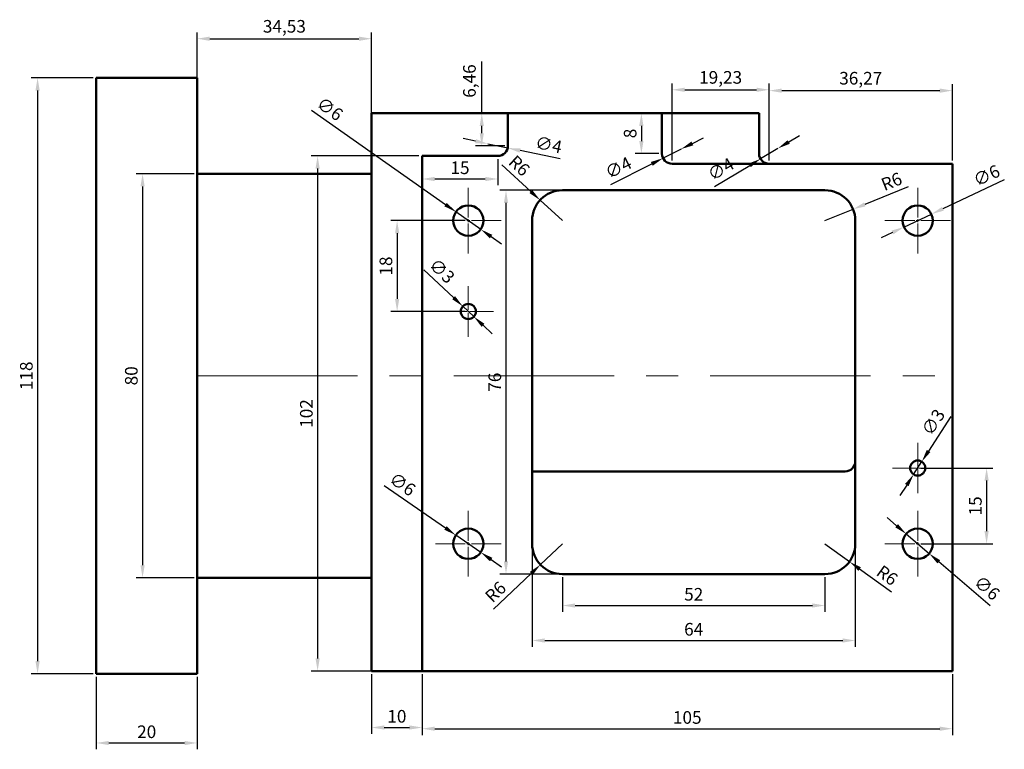
# Model space of a CAD drawing. Units: millimetres. Extents: x 1194 to 1920, y 1729 to 2086.
# Tile 3 of 5: x 1494 to 1689, y 1729 to 1874. Entities that reach past the tile are written whole.
import ezdxf

# ---------------------------------------------------------------- set-up
doc = ezdxf.new("R2010")
doc.units = ezdxf.units.MM
doc.linetypes.add('CENTER', pattern=[50.8, 31.75, -6.35, 6.35, -6.35])
for name, color, linetype, lineweight in [('M-CNTR', 1, 'CENTER', 18), ('M-DIMS', 2, 'Continuous', 25), ('M-OUTL', 7, 'Continuous', 50)]:
    doc.layers.add(name, color=color, linetype=linetype, lineweight=lineweight)
doc.styles.get("Standard").update_dxf_attribs({"font": 'arial.ttf'})
doc.dimstyles.new('ISO-25', dxfattribs={"dimtxt": 2.5, "dimasz": 2.5, "dimexe": 1.25, "dimexo": 0.625, "dimtad": 1, "dimtxsty": 'Standard', "dimcen": 2.5, "dimadec": 0, "dimazin": 0, "dimtfac": 1, "dimtmove": 0, "dimatfit": 3, "dimfxl": 1, "dimarcsym": 0})

# ---------------------------------------------------------------- blocks, each defined once
blk = doc.blocks.new('*D101')
at = {"layer": 'Defpoints', "color": 0, "transparency": 16777216}
for p in [(1509.24, 1862.41), (1497.63, 1744.41), (1509.24, 1744.41)]:
    blk.add_point(p, dxfattribs=at)
at = {"layer": 'M-DIMS', "color": 0, "lineweight": -2, "transparency": 16777216}
for p, q in [((1508.62, 1862.41), (1496.38, 1862.41)), ((1497.63, 1859.91), (1497.63, 1746.91)), ((1508.62, 1744.41), (1496.38, 1744.41))]:
    blk.add_line(p, q, dxfattribs=at)
at = {"layer": 'M-DIMS', "color": 0, "transparency": 16777216}
for points in [[(1497.22, 1859.91), (1498.05, 1859.91), (1497.63, 1862.41)], [(1497.22, 1746.91), (1498.05, 1746.91), (1497.63, 1744.41)]]:
    blk.add_solid(points, dxfattribs=at)
at = {"layer": 'M-DIMS', "color": 0, "transparency": 16777216, "insert": (1495.73, 1803.41), "char_height": 2.5, "attachment_point": 5, "rotation": 90}
blk.add_mtext('118', dxfattribs=at)
blk = doc.blocks.new('*D102')
at = {"layer": 'Defpoints', "color": 0, "transparency": 16777216}
for p in [(1509.24, 1744.41), (1529.24, 1744.41), (1529.24, 1730.7)]:
    blk.add_point(p, dxfattribs=at)
at = {"layer": 'M-DIMS', "color": 0, "lineweight": -2, "transparency": 16777216}
for p, q in [((1509.24, 1743.78), (1509.24, 1729.45)), ((1529.24, 1743.78), (1529.24, 1729.45)), ((1511.74, 1730.7), (1526.74, 1730.7))]:
    blk.add_line(p, q, dxfattribs=at)
at = {"layer": 'M-DIMS', "color": 0, "transparency": 16777216}
for points in [[(1511.74, 1731.11), (1511.74, 1730.28), (1509.24, 1730.7)], [(1526.74, 1731.11), (1526.74, 1730.28), (1529.24, 1730.7)]]:
    blk.add_solid(points, dxfattribs=at)
at = {"layer": 'M-DIMS', "color": 0, "transparency": 16777216, "insert": (1519.24, 1732.6), "char_height": 2.5, "attachment_point": 5}
blk.add_mtext('20', dxfattribs=at)
blk = doc.blocks.new('*D103')
at = {"layer": 'Defpoints', "color": 0, "transparency": 16777216}
for p in [(1563.78, 1870.17), (1529.24, 1843.41), (1563.78, 1843.41)]:
    blk.add_point(p, dxfattribs=at)
at = {"layer": 'M-DIMS', "color": 0, "lineweight": -2, "transparency": 16777216}
for p, q in [((1529.24, 1844.03), (1529.24, 1871.42)), ((1531.74, 1870.17), (1561.28, 1870.17)), ((1563.78, 1844.03), (1563.78, 1871.42))]:
    blk.add_line(p, q, dxfattribs=at)
at = {"layer": 'M-DIMS', "color": 0, "transparency": 16777216}
for points in [[(1531.74, 1870.59), (1531.74, 1869.75), (1529.24, 1870.17)], [(1561.28, 1870.59), (1561.28, 1869.75), (1563.78, 1870.17)]]:
    blk.add_solid(points, dxfattribs=at)
at = {"layer": 'M-DIMS', "color": 0, "transparency": 16777216, "insert": (1546.51, 1872.3), "char_height": 2.5, "attachment_point": 5}
blk.add_mtext('34,53', dxfattribs=at)
blk = doc.blocks.new('*D104')
at = {"layer": 'Defpoints', "color": 0, "transparency": 16777216}
for p in [(1529.24, 1843.41), (1518.42, 1763.41), (1529.24, 1763.41)]:
    blk.add_point(p, dxfattribs=at)
at = {"layer": 'M-DIMS', "color": 0, "lineweight": -2, "transparency": 16777216}
for p, q in [((1528.62, 1843.41), (1517.17, 1843.41)), ((1518.42, 1840.91), (1518.42, 1765.91)), ((1528.62, 1763.41), (1517.17, 1763.41))]:
    blk.add_line(p, q, dxfattribs=at)
at = {"layer": 'M-DIMS', "color": 0, "transparency": 16777216}
for points in [[(1518.01, 1840.91), (1518.84, 1840.91), (1518.42, 1843.41)], [(1518.01, 1765.91), (1518.84, 1765.91), (1518.42, 1763.41)]]:
    blk.add_solid(points, dxfattribs=at)
at = {"layer": 'M-DIMS', "color": 0, "transparency": 16777216, "insert": (1516.52, 1803.41), "char_height": 2.5, "attachment_point": 5, "rotation": 90}
blk.add_mtext('80', dxfattribs=at)
blk = doc.blocks.new('*D105')
at = {"layer": 'Defpoints', "color": 0, "transparency": 16777216}
for p in [(1563.78, 1744.95), (1573.78, 1744.95), (1573.78, 1733.76)]:
    blk.add_point(p, dxfattribs=at)
at = {"layer": 'M-DIMS', "color": 0, "lineweight": -2, "transparency": 16777216}
for p, q in [((1563.78, 1744.32), (1563.78, 1732.51)), ((1573.78, 1744.32), (1573.78, 1732.51)), ((1566.28, 1733.76), (1571.28, 1733.76))]:
    blk.add_line(p, q, dxfattribs=at)
at = {"layer": 'M-DIMS', "color": 0, "transparency": 16777216}
for points in [[(1566.28, 1734.18), (1566.28, 1733.35), (1563.78, 1733.76)], [(1571.28, 1734.18), (1571.28, 1733.35), (1573.78, 1733.76)]]:
    blk.add_solid(points, dxfattribs=at)
at = {"layer": 'M-DIMS', "color": 0, "transparency": 16777216, "insert": (1568.78, 1735.66), "char_height": 2.5, "attachment_point": 5}
blk.add_mtext('10', dxfattribs=at)
blk = doc.blocks.new('*D106')
at = {"layer": 'Defpoints', "color": 0, "transparency": 16777216}
for p in [(1573.78, 1744.95), (1678.78, 1744.95), (1678.78, 1733.53)]:
    blk.add_point(p, dxfattribs=at)
at = {"layer": 'M-DIMS', "color": 0, "lineweight": -2, "transparency": 16777216}
for p, q in [((1573.78, 1744.32), (1573.78, 1732.28)), ((1678.78, 1744.32), (1678.78, 1732.28)), ((1576.28, 1733.53), (1676.28, 1733.53))]:
    blk.add_line(p, q, dxfattribs=at)
at = {"layer": 'M-DIMS', "color": 0, "transparency": 16777216}
for points in [[(1576.28, 1733.95), (1576.28, 1733.11), (1573.78, 1733.53)], [(1676.28, 1733.95), (1676.28, 1733.11), (1678.78, 1733.53)]]:
    blk.add_solid(points, dxfattribs=at)
at = {"layer": 'M-DIMS', "color": 0, "transparency": 16777216, "insert": (1626.28, 1735.43), "char_height": 2.5, "attachment_point": 5}
blk.add_mtext('105', dxfattribs=at)
blk = doc.blocks.new('*D107')
at = {"layer": 'Defpoints', "color": 0, "transparency": 16777216}
for p in [(1573.78, 1846.95), (1553.08, 1744.95), (1573.78, 1744.95)]:
    blk.add_point(p, dxfattribs=at)
at = {"layer": 'M-DIMS', "color": 0, "lineweight": -2, "transparency": 16777216}
for p, q in [((1573.15, 1846.95), (1551.83, 1846.95)), ((1553.08, 1844.45), (1553.08, 1747.45)), ((1573.15, 1744.95), (1551.83, 1744.95))]:
    blk.add_line(p, q, dxfattribs=at)
at = {"layer": 'M-DIMS', "color": 0, "transparency": 16777216}
for points in [[(1552.67, 1844.45), (1553.5, 1844.45), (1553.08, 1846.95)], [(1552.67, 1747.45), (1553.5, 1747.45), (1553.08, 1744.95)]]:
    blk.add_solid(points, dxfattribs=at)
at = {"layer": 'M-DIMS', "color": 0, "transparency": 16777216, "insert": (1551.18, 1795.95), "char_height": 2.5, "attachment_point": 5, "rotation": 90}
blk.add_mtext('102', dxfattribs=at)
blk = doc.blocks.new('*D108')
at = {"layer": 'Defpoints', "color": 0, "transparency": 16777216}
for p in [(1585.59, 1855.41), (1590.78, 1855.41), (1590.78, 1848.95)]:
    blk.add_point(p, dxfattribs=at)
at = {"layer": 'M-DIMS', "color": 0, "lineweight": -2, "transparency": 16777216}
for p, q in [((1585.59, 1855.41), (1585.59, 1865.66)), ((1590.15, 1855.41), (1584.34, 1855.41)), ((1585.59, 1851.45), (1585.59, 1852.91)), ((1590.15, 1848.95), (1584.34, 1848.95))]:
    blk.add_line(p, q, dxfattribs=at)
at = {"layer": 'M-DIMS', "color": 0, "transparency": 16777216}
for points in [[(1585.18, 1852.91), (1586.01, 1852.91), (1585.59, 1855.41)], [(1585.18, 1851.45), (1586.01, 1851.45), (1585.59, 1848.95)]]:
    blk.add_solid(points, dxfattribs=at)
at = {"layer": 'M-DIMS', "color": 0, "transparency": 16777216, "insert": (1583.47, 1861.79), "char_height": 2.5, "attachment_point": 5, "rotation": 90}
blk.add_mtext('6,46', dxfattribs=at)
blk = doc.blocks.new('*D109')
at = {"layer": 'Defpoints', "color": 0, "transparency": 16777216}
for p in [(1573.78, 1846.95), (1588.78, 1846.95), (1588.78, 1842.39)]:
    blk.add_point(p, dxfattribs=at)
at = {"layer": 'M-DIMS', "color": 0, "lineweight": -2, "transparency": 16777216}
for p, q in [((1573.78, 1846.32), (1573.78, 1841.14)), ((1588.78, 1846.32), (1588.78, 1841.14)), ((1576.28, 1842.39), (1586.28, 1842.39))]:
    blk.add_line(p, q, dxfattribs=at)
at = {"layer": 'M-DIMS', "color": 0, "transparency": 16777216}
for points in [[(1576.28, 1842.81), (1576.28, 1841.97), (1573.78, 1842.39)], [(1586.28, 1842.81), (1586.28, 1841.97), (1588.78, 1842.39)]]:
    blk.add_solid(points, dxfattribs=at)
at = {"layer": 'M-DIMS', "color": 0, "transparency": 16777216, "insert": (1581.28, 1844.29), "char_height": 2.5, "attachment_point": 5}
blk.add_mtext('15', dxfattribs=at)
blk = doc.blocks.new('*D110')
at = {"layer": 'Defpoints', "color": 0, "transparency": 16777216}
for p in [(1586.82, 1849.36), (1590.73, 1848.53)]:
    blk.add_point(p, dxfattribs=at)
at = {"layer": 'M-DIMS', "color": 0, "lineweight": -2, "transparency": 16777216}
for p, q in [((1584.37, 1849.87), (1581.93, 1850.39)), ((1586.82, 1849.36), (1590.73, 1848.53)), ((1601.11, 1846.35), (1593.18, 1848.02))]:
    blk.add_line(p, q, dxfattribs=at)
at = {"layer": 'M-DIMS', "color": 0, "transparency": 16777216}
for points in [[(1584.46, 1850.28), (1584.29, 1849.46), (1586.82, 1849.36)], [(1593.27, 1848.43), (1593.1, 1847.61), (1590.73, 1848.53)]]:
    blk.add_solid(points, dxfattribs=at)
at = {"layer": 'M-DIMS', "color": 0, "transparency": 16777216, "insert": (1598.77, 1848.86), "char_height": 2.5, "attachment_point": 5, "rotation": 348.1195}
blk.add_mtext('∅4', dxfattribs=at)
blk = doc.blocks.new('*D111')
at = {"layer": 'Defpoints', "color": 0, "transparency": 16777216}
for p in [(1621.49, 1846.51), (1625.06, 1848.31)]:
    blk.add_point(p, dxfattribs=at)
at = {"layer": 'M-DIMS', "color": 0, "lineweight": -2, "transparency": 16777216}
for p, q in [((1627.3, 1849.43), (1629.53, 1850.55)), ((1625.06, 1848.31), (1621.49, 1846.51)), ((1611.16, 1841.32), (1619.26, 1845.39))]:
    blk.add_line(p, q, dxfattribs=at)
at = {"layer": 'M-DIMS', "color": 0, "transparency": 16777216}
for points in [[(1627.11, 1849.8), (1627.49, 1849.06), (1625.06, 1848.31)], [(1619.07, 1845.76), (1619.44, 1845.01), (1621.49, 1846.51)]]:
    blk.add_solid(points, dxfattribs=at)
at = {"layer": 'M-DIMS', "color": 0, "transparency": 16777216, "insert": (1612.78, 1844.34), "char_height": 2.5, "attachment_point": 5, "rotation": 26.6783}
blk.add_mtext('∅4', dxfattribs=at)
blk = doc.blocks.new('*D112')
at = {"layer": 'Defpoints', "color": 0, "transparency": 16777216}
for p in [(1644.23, 1848.44), (1640.8, 1846.38)]:
    blk.add_point(p, dxfattribs=at)
at = {"layer": 'M-DIMS', "color": 0, "lineweight": -2, "transparency": 16777216}
for p, q in [((1646.37, 1849.72), (1648.52, 1851.01)), ((1644.23, 1848.44), (1640.8, 1846.38)), ((1631.71, 1840.93), (1638.65, 1845.09))]:
    blk.add_line(p, q, dxfattribs=at)
at = {"layer": 'M-DIMS', "color": 0, "transparency": 16777216}
for points in [[(1646.16, 1850.08), (1646.59, 1849.36), (1644.23, 1848.44)], [(1638.44, 1845.45), (1638.87, 1844.74), (1640.8, 1846.38)]]:
    blk.add_solid(points, dxfattribs=at)
at = {"layer": 'M-DIMS', "color": 0, "transparency": 16777216, "insert": (1633.09, 1844.06), "char_height": 2.5, "attachment_point": 5, "rotation": 30.9377}
blk.add_mtext('∅4', dxfattribs=at)
blk = doc.blocks.new('*D113')
at = {"layer": 'Defpoints', "color": 0, "transparency": 16777216}
for p in [(1621.28, 1855.41), (1617.2, 1847.41), (1621.28, 1847.41)]:
    blk.add_point(p, dxfattribs=at)
at = {"layer": 'M-DIMS', "color": 0, "lineweight": -2, "transparency": 16777216}
for p, q in [((1620.65, 1855.41), (1615.95, 1855.41)), ((1617.2, 1852.91), (1617.2, 1849.91)), ((1620.65, 1847.41), (1615.95, 1847.41))]:
    blk.add_line(p, q, dxfattribs=at)
at = {"layer": 'M-DIMS', "color": 0, "transparency": 16777216}
for points in [[(1616.78, 1852.91), (1617.62, 1852.91), (1617.2, 1855.41)], [(1616.78, 1849.91), (1617.62, 1849.91), (1617.2, 1847.41)]]:
    blk.add_solid(points, dxfattribs=at)
at = {"layer": 'M-DIMS', "color": 0, "transparency": 16777216, "insert": (1615.3, 1851.41), "char_height": 2.5, "attachment_point": 5, "rotation": 90}
blk.add_mtext('8', dxfattribs=at)
blk = doc.blocks.new('*D114')
at = {"layer": 'Defpoints', "color": 0, "transparency": 16777216}
for p in [(1642.51, 1860.06), (1623.28, 1845.41), (1642.51, 1845.41)]:
    blk.add_point(p, dxfattribs=at)
at = {"layer": 'M-DIMS', "color": 0, "lineweight": -2, "transparency": 16777216}
for p, q in [((1623.28, 1846.03), (1623.28, 1861.31)), ((1642.51, 1846.03), (1642.51, 1861.31)), ((1625.78, 1860.06), (1640.01, 1860.06))]:
    blk.add_line(p, q, dxfattribs=at)
at = {"layer": 'M-DIMS', "color": 0, "transparency": 16777216}
for points in [[(1625.78, 1860.48), (1625.78, 1859.64), (1623.28, 1860.06)], [(1640.01, 1860.48), (1640.01, 1859.64), (1642.51, 1860.06)]]:
    blk.add_solid(points, dxfattribs=at)
at = {"layer": 'M-DIMS', "color": 0, "transparency": 16777216, "insert": (1632.89, 1862.19), "char_height": 2.5, "attachment_point": 5}
blk.add_mtext('19,23', dxfattribs=at)
blk = doc.blocks.new('*D115')
at = {"layer": 'Defpoints', "color": 0, "transparency": 16777216}
for p in [(1678.78, 1859.89), (1642.51, 1845.41), (1678.78, 1845.41)]:
    blk.add_point(p, dxfattribs=at)
at = {"layer": 'M-DIMS', "color": 0, "lineweight": -2, "transparency": 16777216}
for p, q in [((1642.51, 1846.03), (1642.51, 1861.14)), ((1678.78, 1846.03), (1678.78, 1861.14)), ((1645.01, 1859.89), (1676.28, 1859.89))]:
    blk.add_line(p, q, dxfattribs=at)
at = {"layer": 'M-DIMS', "color": 0, "transparency": 16777216}
for points in [[(1645.01, 1860.31), (1645.01, 1859.47), (1642.51, 1859.89)], [(1676.28, 1860.31), (1676.28, 1859.47), (1678.78, 1859.89)]]:
    blk.add_solid(points, dxfattribs=at)
at = {"layer": 'M-DIMS', "color": 0, "transparency": 16777216, "insert": (1660.64, 1862.02), "char_height": 2.5, "attachment_point": 5}
blk.add_mtext('36,27', dxfattribs=at)
blk = doc.blocks.new('*D116')
at = {"layer": 'Defpoints', "color": 0, "transparency": 16777216}
for p in [(1601.56, 1764.15), (1653.56, 1764.15), (1653.56, 1757.92)]:
    blk.add_point(p, dxfattribs=at)
at = {"layer": 'M-DIMS', "color": 0, "lineweight": -2, "transparency": 16777216}
for p, q in [((1601.56, 1763.53), (1601.56, 1756.67)), ((1653.56, 1763.53), (1653.56, 1756.67)), ((1604.06, 1757.92), (1651.06, 1757.92))]:
    blk.add_line(p, q, dxfattribs=at)
at = {"layer": 'M-DIMS', "color": 0, "transparency": 16777216}
for points in [[(1604.06, 1758.34), (1604.06, 1757.51), (1601.56, 1757.92)], [(1651.06, 1758.34), (1651.06, 1757.51), (1653.56, 1757.92)]]:
    blk.add_solid(points, dxfattribs=at)
at = {"layer": 'M-DIMS', "color": 0, "transparency": 16777216, "insert": (1627.56, 1759.82), "char_height": 2.5, "attachment_point": 5}
blk.add_mtext('52', dxfattribs=at)
blk = doc.blocks.new('*D117')
at = {"layer": 'Defpoints', "color": 0, "transparency": 16777216}
for p in [(1595.56, 1770.15), (1659.56, 1770.15), (1659.56, 1751)]:
    blk.add_point(p, dxfattribs=at)
at = {"layer": 'M-DIMS', "color": 0, "lineweight": -2, "transparency": 16777216}
for p, q in [((1595.56, 1769.53), (1595.56, 1749.75)), ((1659.56, 1769.53), (1659.56, 1749.75)), ((1598.06, 1751), (1657.06, 1751))]:
    blk.add_line(p, q, dxfattribs=at)
at = {"layer": 'M-DIMS', "color": 0, "transparency": 16777216}
for points in [[(1598.06, 1751.41), (1598.06, 1750.58), (1595.56, 1751)], [(1657.06, 1751.41), (1657.06, 1750.58), (1659.56, 1751)]]:
    blk.add_solid(points, dxfattribs=at)
at = {"layer": 'M-DIMS', "color": 0, "transparency": 16777216, "insert": (1627.56, 1752.9), "char_height": 2.5, "attachment_point": 5}
blk.add_mtext('64', dxfattribs=at)
blk = doc.blocks.new('*D118')
at = {"layer": 'Defpoints', "color": 0, "transparency": 16777216}
for p in [(1601.56, 1840.15), (1590.39, 1764.15), (1601.56, 1764.15)]:
    blk.add_point(p, dxfattribs=at)
at = {"layer": 'M-DIMS', "color": 0, "lineweight": -2, "transparency": 16777216}
for p, q in [((1600.93, 1840.15), (1589.14, 1840.15)), ((1590.39, 1837.65), (1590.39, 1766.65)), ((1600.93, 1764.15), (1589.14, 1764.15))]:
    blk.add_line(p, q, dxfattribs=at)
at = {"layer": 'M-DIMS', "color": 0, "transparency": 16777216}
for points in [[(1589.97, 1837.65), (1590.8, 1837.65), (1590.39, 1840.15)], [(1589.97, 1766.65), (1590.8, 1766.65), (1590.39, 1764.15)]]:
    blk.add_solid(points, dxfattribs=at)
at = {"layer": 'M-DIMS', "color": 0, "transparency": 16777216, "insert": (1588.49, 1802.15), "char_height": 2.5, "attachment_point": 5, "rotation": 90}
blk.add_mtext('76', dxfattribs=at)
blk = doc.blocks.new('*D119')
at = {"layer": 'Defpoints', "color": 0, "transparency": 16777216}
for p in [(1653.56, 1770.15), (1658.4, 1766.61)]:
    blk.add_point(p, dxfattribs=at)
at = {"layer": 'M-DIMS', "color": 0, "lineweight": -2, "transparency": 16777216}
for p, q in [((1653.56, 1770.15), (1658.4, 1766.61)), ((1666.71, 1760.55), (1660.42, 1765.14))]:
    blk.add_line(p, q, dxfattribs=at)
at = {"layer": 'M-DIMS', "color": 0, "transparency": 16777216}
blk.add_solid([(1660.67, 1765.48), (1660.18, 1764.8), (1658.4, 1766.61)], dxfattribs=at)
at = {"layer": 'M-DIMS', "color": 0, "transparency": 16777216, "insert": (1665.69, 1763.64), "char_height": 2.5, "attachment_point": 5, "rotation": 323.8624}
blk.add_mtext('R6', dxfattribs=at)
blk = doc.blocks.new('*D120')
at = {"layer": 'Defpoints', "color": 0, "transparency": 16777216}
for p in [(1601.56, 1770.15), (1597.21, 1766.02)]:
    blk.add_point(p, dxfattribs=at)
at = {"layer": 'M-DIMS', "color": 0, "lineweight": -2, "transparency": 16777216}
for p, q in [((1601.56, 1770.15), (1597.21, 1766.02)), ((1587.93, 1757.19), (1595.4, 1764.29))]:
    blk.add_line(p, q, dxfattribs=at)
at = {"layer": 'M-DIMS', "color": 0, "transparency": 16777216}
blk.add_solid([(1595.11, 1764.59), (1595.69, 1763.99), (1597.21, 1766.02)], dxfattribs=at)
at = {"layer": 'M-DIMS', "color": 0, "transparency": 16777216, "insert": (1588.54, 1760.38), "char_height": 2.5, "attachment_point": 5, "rotation": 43.5809}
blk.add_mtext('R6', dxfattribs=at)
blk = doc.blocks.new('*D121')
at = {"layer": 'Defpoints', "color": 0, "transparency": 16777216}
for p in [(1659.12, 1836.41), (1653.56, 1834.15)]:
    blk.add_point(p, dxfattribs=at)
at = {"layer": 'M-DIMS', "color": 0, "lineweight": -2, "transparency": 16777216}
for p, q in [((1670.03, 1840.83), (1661.44, 1837.35)), ((1653.56, 1834.15), (1659.12, 1836.41))]:
    blk.add_line(p, q, dxfattribs=at)
at = {"layer": 'M-DIMS', "color": 0, "transparency": 16777216}
blk.add_solid([(1661.28, 1837.73), (1661.59, 1836.96), (1659.12, 1836.41)], dxfattribs=at)
at = {"layer": 'M-DIMS', "color": 0, "transparency": 16777216, "insert": (1666.86, 1841.6), "char_height": 2.5, "attachment_point": 5, "rotation": 22.0655}
blk.add_mtext('R6', dxfattribs=at)
blk = doc.blocks.new('*D122')
at = {"layer": 'Defpoints', "color": 0, "transparency": 16777216}
for p in [(1597.14, 1838.21), (1601.56, 1834.15)]:
    blk.add_point(p, dxfattribs=at)
at = {"layer": 'M-DIMS', "color": 0, "lineweight": -2, "transparency": 16777216}
for p, q in [((1589.58, 1845.17), (1595.3, 1839.91)), ((1601.56, 1834.15), (1597.14, 1838.21))]:
    blk.add_line(p, q, dxfattribs=at)
at = {"layer": 'M-DIMS', "color": 0, "transparency": 16777216}
blk.add_solid([(1595.58, 1840.21), (1595.02, 1839.6), (1597.14, 1838.21)], dxfattribs=at)
at = {"layer": 'M-DIMS', "color": 0, "transparency": 16777216, "insert": (1592.81, 1844.79), "char_height": 2.5, "attachment_point": 5, "rotation": 317.3909}
blk.add_mtext('R6', dxfattribs=at)
blk = doc.blocks.new('*U123')
at = {"layer": 'M-CNTR', "color": 0, "transparency": 16777216}
for p, q in [((0, 0.6), (0, 6.5)), ((-6.5, 0), (-0.6, 0)), ((0.6, 0), (6.5, 0)), ((0, -6.5), (0, -0.6))]:
    blk.add_line(p, q, dxfattribs=at)
at = {"layer": 'M-CNTR', "color": 0, "linetype": 'Continuous', "transparency": 16777216}
for p, q in [((-0.3, 0), (0.3, 0)), ((0, -0.3), (0, 0.3))]:
    blk.add_line(p, q, dxfattribs=at)
blk = doc.blocks.new('*U124')
at = {"layer": 'M-CNTR', "color": 0, "transparency": 16777216}
for p, q in [((0, 0.3), (0, 5)), ((-5, 0), (-0.3, 0)), ((0.3, 0), (5, 0)), ((0, -5), (0, -0.3))]:
    blk.add_line(p, q, dxfattribs=at)
at = {"layer": 'M-CNTR', "color": 0, "linetype": 'Continuous', "transparency": 16777216}
for p, q in [((-0.15, 0), (0.15, 0)), ((0, -0.15), (0, 0.15))]:
    blk.add_line(p, q, dxfattribs=at)
blk = doc.blocks.new('*U125')
at = {"layer": 'M-CNTR', "color": 0, "transparency": 16777216}
for p, q in [((0, 0.6), (0, 6.5)), ((-6.5, 0), (-0.6, 0)), ((0.6, 0), (6.5, 0)), ((0, -6.5), (0, -0.6))]:
    blk.add_line(p, q, dxfattribs=at)
at = {"layer": 'M-CNTR', "color": 0, "linetype": 'Continuous', "transparency": 16777216}
for p, q in [((-0.3, 0), (0.3, 0)), ((0, -0.3), (0, 0.3))]:
    blk.add_line(p, q, dxfattribs=at)
blk = doc.blocks.new('*U126')
at = {"layer": 'M-CNTR', "color": 0, "transparency": 16777216}
for p, q in [((0, 0.6), (0, 6.5)), ((-6.5, 0), (-0.6, 0)), ((0.6, 0), (6.5, 0)), ((0, -6.5), (0, -0.6))]:
    blk.add_line(p, q, dxfattribs=at)
at = {"layer": 'M-CNTR', "color": 0, "linetype": 'Continuous', "transparency": 16777216}
for p, q in [((-0.3, 0), (0.3, 0)), ((0, -0.3), (0, 0.3))]:
    blk.add_line(p, q, dxfattribs=at)
blk = doc.blocks.new('*U127')
at = {"layer": 'M-CNTR', "color": 0, "transparency": 16777216}
for p, q in [((0, 0.3), (0, 5)), ((-5, 0), (-0.3, 0)), ((0.3, 0), (5, 0)), ((0, -5), (0, -0.3))]:
    blk.add_line(p, q, dxfattribs=at)
at = {"layer": 'M-CNTR', "color": 0, "linetype": 'Continuous', "transparency": 16777216}
for p, q in [((-0.15, 0), (0.15, 0)), ((0, -0.15), (0, 0.15))]:
    blk.add_line(p, q, dxfattribs=at)
blk = doc.blocks.new('*U128')
at = {"layer": 'M-CNTR', "color": 0, "transparency": 16777216}
for p, q in [((0, 0.6), (0, 6.5)), ((-6.5, 0), (-0.6, 0)), ((0.6, 0), (6.5, 0)), ((0, -6.5), (0, -0.6))]:
    blk.add_line(p, q, dxfattribs=at)
at = {"layer": 'M-CNTR', "color": 0, "linetype": 'Continuous', "transparency": 16777216}
for p, q in [((-0.3, 0), (0.3, 0)), ((0, -0.3), (0, 0.3))]:
    blk.add_line(p, q, dxfattribs=at)
blk = doc.blocks.new('*D129')
at = {"layer": 'Defpoints', "color": 0, "transparency": 16777216}
for p in [(1582.93, 1834.15), (1568.83, 1816.15), (1582.93, 1816.15)]:
    blk.add_point(p, dxfattribs=at)
at = {"layer": 'M-DIMS', "color": 0, "lineweight": -2, "transparency": 16777216}
for p, q in [((1582.31, 1834.15), (1567.58, 1834.15)), ((1568.83, 1831.65), (1568.83, 1818.65)), ((1582.31, 1816.15), (1567.58, 1816.15))]:
    blk.add_line(p, q, dxfattribs=at)
at = {"layer": 'M-DIMS', "color": 0, "transparency": 16777216}
for points in [[(1568.42, 1831.65), (1569.25, 1831.65), (1568.83, 1834.15)], [(1568.42, 1818.65), (1569.25, 1818.65), (1568.83, 1816.15)]]:
    blk.add_solid(points, dxfattribs=at)
at = {"layer": 'M-DIMS', "color": 0, "transparency": 16777216, "insert": (1566.93, 1825.15), "char_height": 2.5, "attachment_point": 5, "rotation": 90}
blk.add_mtext('18', dxfattribs=at)
blk = doc.blocks.new('*D130')
at = {"layer": 'Defpoints', "color": 0, "transparency": 16777216}
for p in [(1671.92, 1785.15), (1671.92, 1770.15), (1685.56, 1770.15)]:
    blk.add_point(p, dxfattribs=at)
at = {"layer": 'M-DIMS', "color": 0, "lineweight": -2, "transparency": 16777216}
for p, q in [((1672.54, 1785.15), (1686.81, 1785.15)), ((1685.56, 1782.65), (1685.56, 1772.65)), ((1672.54, 1770.15), (1686.81, 1770.15))]:
    blk.add_line(p, q, dxfattribs=at)
at = {"layer": 'M-DIMS', "color": 0, "transparency": 16777216}
for points in [[(1685.14, 1782.65), (1685.98, 1782.65), (1685.56, 1785.15)], [(1685.14, 1772.65), (1685.98, 1772.65), (1685.56, 1770.15)]]:
    blk.add_solid(points, dxfattribs=at)
at = {"layer": 'M-DIMS', "color": 0, "transparency": 16777216, "insert": (1683.66, 1777.65), "char_height": 2.5, "attachment_point": 5, "rotation": 90}
blk.add_mtext('15', dxfattribs=at)
blk = doc.blocks.new('*D131')
at = {"layer": 'Defpoints', "color": 0, "transparency": 16777216}
for p in [(1580.48, 1835.88), (1585.38, 1832.42)]:
    blk.add_point(p, dxfattribs=at)
at = {"layer": 'M-DIMS', "color": 0, "lineweight": -2, "transparency": 16777216}
for p, q in [((1551.89, 1856.01), (1578.43, 1837.32)), ((1585.38, 1832.42), (1580.48, 1835.88)), ((1587.43, 1830.99), (1589.47, 1829.55))]:
    blk.add_line(p, q, dxfattribs=at)
at = {"layer": 'M-DIMS', "color": 0, "transparency": 16777216}
for points in [[(1578.67, 1837.66), (1578.19, 1836.98), (1580.48, 1835.88)], [(1587.67, 1831.33), (1587.19, 1830.64), (1585.38, 1832.42)]]:
    blk.add_solid(points, dxfattribs=at)
at = {"layer": 'M-DIMS', "color": 0, "transparency": 16777216, "insert": (1555.32, 1856), "char_height": 2.5, "attachment_point": 5, "rotation": 324.8513}
blk.add_mtext('∅6', dxfattribs=at)
blk = doc.blocks.new('*D132')
at = {"layer": 'Defpoints', "color": 0, "transparency": 16777216}
for p in [(1581.84, 1817.18), (1584.03, 1815.13)]:
    blk.add_point(p, dxfattribs=at)
at = {"layer": 'M-DIMS', "color": 0, "lineweight": -2, "transparency": 16777216}
for p, q in [((1574.09, 1824.43), (1580.01, 1818.89)), ((1584.03, 1815.13), (1581.84, 1817.18)), ((1585.85, 1813.42), (1587.67, 1811.71))]:
    blk.add_line(p, q, dxfattribs=at)
at = {"layer": 'M-DIMS', "color": 0, "transparency": 16777216}
for points in [[(1580.3, 1819.19), (1579.73, 1818.58), (1581.84, 1817.18)], [(1586.13, 1813.72), (1585.56, 1813.11), (1584.03, 1815.13)]]:
    blk.add_solid(points, dxfattribs=at)
at = {"layer": 'M-DIMS', "color": 0, "transparency": 16777216, "insert": (1577.49, 1823.95), "char_height": 2.5, "attachment_point": 5, "rotation": 316.8666}
blk.add_mtext('∅3', dxfattribs=at)
blk = doc.blocks.new('*D133')
at = {"layer": 'Defpoints', "color": 0, "transparency": 16777216}
for p in [(1580.46, 1771.86), (1585.4, 1768.45)]:
    blk.add_point(p, dxfattribs=at)
at = {"layer": 'M-DIMS', "color": 0, "lineweight": -2, "transparency": 16777216}
for p, q in [((1566.28, 1781.67), (1578.41, 1773.28)), ((1585.4, 1768.45), (1580.46, 1771.86)), ((1587.45, 1767.02), (1589.51, 1765.6))]:
    blk.add_line(p, q, dxfattribs=at)
at = {"layer": 'M-DIMS', "color": 0, "transparency": 16777216}
for points in [[(1578.64, 1773.62), (1578.17, 1772.94), (1580.46, 1771.86)], [(1587.69, 1767.37), (1587.22, 1766.68), (1585.4, 1768.45)]]:
    blk.add_solid(points, dxfattribs=at)
at = {"layer": 'M-DIMS', "color": 0, "transparency": 16777216, "insert": (1569.7, 1781.69), "char_height": 2.5, "attachment_point": 5, "rotation": 325.3406}
blk.add_mtext('∅6', dxfattribs=at)
blk = doc.blocks.new('*D134')
at = {"layer": 'Defpoints', "color": 0, "transparency": 16777216}
for p in [(1669.64, 1772.1), (1674.2, 1768.2)]:
    blk.add_point(p, dxfattribs=at)
at = {"layer": 'M-DIMS', "color": 0, "lineweight": -2, "transparency": 16777216}
for p, q in [((1667.74, 1773.73), (1665.84, 1775.36)), ((1669.64, 1772.1), (1674.2, 1768.2)), ((1686.28, 1757.85), (1676.09, 1766.57))]:
    blk.add_line(p, q, dxfattribs=at)
at = {"layer": 'M-DIMS', "color": 0, "transparency": 16777216}
for points in [[(1668.01, 1774.05), (1667.47, 1773.41), (1669.64, 1772.1)], [(1676.37, 1766.89), (1675.82, 1766.26), (1674.2, 1768.2)]]:
    blk.add_solid(points, dxfattribs=at)
at = {"layer": 'M-DIMS', "color": 0, "transparency": 16777216, "insert": (1685.43, 1761.17), "char_height": 2.5, "attachment_point": 5, "rotation": 319.4213}
blk.add_mtext('∅6', dxfattribs=at)
blk = doc.blocks.new('*D135')
at = {"layer": 'Defpoints', "color": 0, "transparency": 16777216}
for p in [(1672.73, 1786.42), (1671.11, 1783.89)]:
    blk.add_point(p, dxfattribs=at)
at = {"layer": 'M-DIMS', "color": 0, "lineweight": -2, "transparency": 16777216}
for p, q in [((1678.45, 1795.35), (1674.07, 1788.52)), ((1671.11, 1783.89), (1672.73, 1786.42)), ((1669.76, 1781.78), (1668.41, 1779.68))]:
    blk.add_line(p, q, dxfattribs=at)
at = {"layer": 'M-DIMS', "color": 0, "transparency": 16777216}
for points in [[(1673.72, 1788.75), (1674.42, 1788.3), (1672.73, 1786.42)], [(1669.41, 1782.01), (1670.11, 1781.56), (1671.11, 1783.89)]]:
    blk.add_solid(points, dxfattribs=at)
at = {"layer": 'M-DIMS', "color": 0, "transparency": 16777216, "insert": (1675.27, 1794.05), "char_height": 2.5, "attachment_point": 5, "rotation": 57.3649}
blk.add_mtext('∅3', dxfattribs=at)
blk = doc.blocks.new('*D136')
at = {"layer": 'Defpoints', "color": 0, "transparency": 16777216}
for p in [(1674.63, 1835.43), (1669.2, 1832.88)]:
    blk.add_point(p, dxfattribs=at)
at = {"layer": 'M-DIMS', "color": 0, "lineweight": -2, "transparency": 16777216}
for p, q in [((1689.07, 1842.2), (1676.9, 1836.49)), ((1669.2, 1832.88), (1674.63, 1835.43)), ((1666.94, 1831.82), (1664.67, 1830.75))]:
    blk.add_line(p, q, dxfattribs=at)
at = {"layer": 'M-DIMS', "color": 0, "transparency": 16777216}
for points in [[(1676.72, 1836.86), (1677.07, 1836.11), (1674.63, 1835.43)], [(1666.76, 1832.19), (1667.11, 1831.44), (1669.2, 1832.88)]]:
    blk.add_solid(points, dxfattribs=at)
at = {"layer": 'M-DIMS', "color": 0, "transparency": 16777216, "insert": (1685.69, 1842.79), "char_height": 2.5, "attachment_point": 5, "rotation": 25.1264}
blk.add_mtext('∅6', dxfattribs=at)

msp = doc.modelspace()

# ---------------------------------------------------------------- linework, layer by layer
at = {"layer": 'M-CNTR'}
msp.add_line((1529.2434, 1803.4077), (1678.7776, 1803.4077), dxfattribs=at)
at = {"layer": 'M-OUTL'}
for p, q in [((1509.2434, 1862.4077), (1509.2434, 1744.4077)), ((1529.2434, 1862.4077), (1509.2434, 1862.4077)), ((1529.2434, 1744.4077), (1529.2434, 1862.4077)), ((1563.7776, 1843.4077), (1563.7776, 1855.4077)), ((1563.7776, 1855.4077), (1640.5117, 1855.4077)), ((1590.7776, 1848.9456), (1590.7776, 1855.4077)), ((1590.7776, 1855.4077), (1621.2776, 1855.4077)), ((1621.2776, 1855.4077), (1621.2776, 1847.4077)), ((1640.5117, 1855.4077), (1640.5117, 1847.4077)), ((1573.7776, 1744.9456), (1573.7776, 1846.9456)), ((1573.7776, 1846.9456), (1588.7776, 1846.9456)), ((1623.2776, 1845.4077), (1642.5117, 1845.4077)), ((1642.5117, 1845.4077), (1678.7776, 1845.4077)), ((1678.7776, 1845.4077), (1678.7776, 1744.9456)), ((1529.2434, 1803.4077), (1529.2434, 1843.4077)), ((1529.2434, 1843.4077), (1563.7776, 1843.4077)), ((1563.7776, 1843.4077), (1563.7776, 1763.4077)), ((1653.5579, 1840.1519), (1601.5579, 1840.1519)), ((1595.5579, 1834.1519), (1595.5579, 1770.1519)), ((1659.5579, 1786.4732), (1659.5579, 1834.1519)), ((1659.5579, 1786.4732), (1659.5579, 1770.1519)), ((1595.5579, 1784.4732), (1657.5579, 1784.4732)), ((1563.7776, 1763.4077), (1529.2434, 1763.4077)), ((1563.7776, 1744.9456), (1563.7776, 1763.4077)), ((1601.5579, 1764.1519), (1653.5579, 1764.1519)), ((1509.2434, 1744.4077), (1529.2434, 1744.4077)), ((1678.7776, 1744.9456), (1563.7776, 1744.9456)), ((1563.7776, 1744.9456), (1573.7776, 1744.9456))]:
    msp.add_line(p, q, dxfattribs=at)
for centre, radius in [((1582.9306, 1834.1519), 3), ((1671.9167, 1834.1519), 3), ((1582.9306, 1816.1519), 1.5), ((1671.9167, 1785.1519), 1.5), ((1582.9306, 1770.1519), 3), ((1671.9167, 1770.1519), 3)]:
    msp.add_circle(centre, radius, dxfattribs=at)
for centre, radius, start, end in [((1588.7776, 1848.9456), 2, 270, 0), ((1623.2776, 1847.4077), 2, 180, 270), ((1642.5117, 1847.4077), 2, 180, 270), ((1601.5579, 1834.1519), 6, 90, 180), ((1653.5579, 1834.1519), 6, 0, 90), ((1657.5579, 1786.4732), 2, 270, 0), ((1601.5579, 1770.1519), 6, 180, 270), ((1653.5579, 1770.1519), 6, 270, 0)]:
    msp.add_arc(centre, radius, start, end, dxfattribs=at)

# ---------------------------------------------------------------- block references
at = {"layer": 'M-CNTR'}
for name, p in [('*U123', (1582.9306, 1834.1519)), ('*U128', (1671.9167, 1834.1519)), ('*U124', (1582.9306, 1816.1519)), ('*U127', (1671.9167, 1785.1519)), ('*U125', (1582.9306, 1770.1519)), ('*U126', (1671.9167, 1770.1519))]:
    msp.add_blockref(name, p, dxfattribs=at)

# ---------------------------------------------------------------- dimensions: what is measured, and where the dimension line sits
at = {"layer": 'M-DIMS'}
for base, p1, p2, picture, middle in [((1563.7776, 1870.1702), (1529.2434, 1843.4077), (1563.7776, 1843.4077), '*D103', (1546.5105, 1872.2976)), ((1642.5117, 1860.0603), (1623.2776, 1845.4077), (1642.5117, 1845.4077), '*D114', (1632.8946, 1862.1877)), ((1678.7776, 1859.8892), (1642.5117, 1845.4077), (1678.7776, 1845.4077), '*D115', (1660.6446, 1862.0166)), ((1588.7776, 1842.3897), (1573.7776, 1846.9456), (1588.7776, 1846.9456), '*D109', (1581.2776, 1844.2911)), ((1659.5579, 1750.9953), (1595.5579, 1770.1519), (1659.5579, 1770.1519), '*D117', (1627.5579, 1752.8968)), ((1653.5579, 1757.9229), (1601.5579, 1764.1519), (1653.5579, 1764.1519), '*D116', (1627.5579, 1759.8243)), ((1529.2434, 1730.6974), (1509.2434, 1744.4077), (1529.2434, 1744.4077), '*D102', (1519.2434, 1732.5988)), ((1573.7776, 1733.7623), (1563.7776, 1744.9456), (1573.7776, 1744.9456), '*D105', (1568.7776, 1735.6637)), ((1678.7776, 1733.5287), (1573.7776, 1744.9456), (1678.7776, 1744.9456), '*D106', (1626.2776, 1735.4301))]:
    dim = msp.add_linear_dim(base=base, p1=p1, p2=p2, dimstyle='ISO-25', override={"dimclrd": 0, "dimclre": 0, "dimclrt": 0}, dxfattribs=at)
    dim.commit()
    dim.dimension.update_dxf_attribs({"geometry": picture, "text_midpoint": middle})
for base, p1, p2, picture, middle in [((1585.5945, 1855.4077), (1590.7776, 1848.9456), (1590.7776, 1855.4077), '*D108', (1583.4671, 1861.7856)), ((1497.6327, 1744.4077), (1509.2434, 1862.4077), (1509.2434, 1744.4077), '*D101', (1495.7313, 1803.4077)), ((1617.1983, 1847.4077), (1621.2776, 1855.4077), (1621.2776, 1847.4077), '*D113', (1615.2969, 1851.4077)), ((1553.0825, 1744.9456), (1573.7776, 1846.9456), (1573.7776, 1744.9456), '*D107', (1551.181, 1795.9456)), ((1518.4234, 1763.4077), (1529.2434, 1843.4077), (1529.2434, 1763.4077), '*D104', (1516.522, 1803.4077)), ((1590.3874, 1764.1519), (1601.5579, 1840.1519), (1601.5579, 1764.1519), '*D118', (1588.4859, 1802.1519)), ((1568.8347, 1816.1519), (1582.9306, 1834.1519), (1582.9306, 1816.1519), '*D129', (1566.9332, 1825.1519)), ((1685.5608, 1770.1519), (1671.9167, 1785.1519), (1671.9167, 1770.1519), '*D130', (1683.6594, 1777.6519))]:
    dim = msp.add_linear_dim(base=base, p1=p1, p2=p2, angle=90, dimstyle='ISO-25', override={"dimclrd": 0, "dimclre": 0, "dimclrt": 0}, dxfattribs=at)
    dim.commit()
    dim.dimension.update_dxf_attribs({"geometry": picture, "text_midpoint": middle})
for p1, p2, picture, middle in [((1585.3836, 1832.4248), (1580.4776, 1835.879), '*D131', (1554.1829, 1854.3927)), ((1625.0646, 1848.3057), (1621.4905, 1846.5097), '*D111', (1613.6611, 1842.5757)), ((1669.2006, 1832.8781), (1674.6328, 1835.4258), '*D136', (1686.5294, 1841.0052)), ((1585.3982, 1768.4458), (1580.463, 1771.858), '*D133', (1568.5811, 1780.073)), ((1669.6382, 1772.1034), (1674.1953, 1768.2005), '*D134', (1684.1466, 1759.6775))]:
    dim = msp.add_diameter_dim_2p(p1=p1, p2=p2, dimstyle='ISO-25', override={"dimclrd": 0, "dimclre": 0, "dimclrt": 0}, dxfattribs=at)
    dim.commit()
    dim.dimension.update_dxf_attribs({"geometry": picture, "text_midpoint": middle, "dimtype": 163})
for p1, p2, picture, middle in [((1586.8204, 1849.3574), (1590.7347, 1848.5339), '*D110', (1598.7728, 1848.8574)), ((1644.2271, 1848.4359), (1640.7962, 1846.3795), '*D112', (1633.0931, 1844.0607)), ((1584.0252, 1815.1264), (1581.8359, 1817.1775), '*D132', (1577.4884, 1823.952)), ((1671.1078, 1783.8887), (1672.7256, 1786.4151), '*D135', (1675.2743, 1794.0505))]:
    dim = msp.add_diameter_dim_2p(p1=p1, p2=p2, dimstyle='ISO-25', override={"dimclrd": 0, "dimclre": 0, "dimclrt": 0}, dxfattribs=at)
    dim.commit()
    dim.dimension.update_dxf_attribs({"geometry": picture, "text_midpoint": middle})
for center, mpoint, picture, middle in [((1601.5579, 1834.1519), (1597.142, 1838.2139), '*D122', (1592.8064, 1844.7854)), ((1653.5579, 1770.1519), (1658.4035, 1766.6136), '*D119', (1665.6948, 1763.6438))]:
    dim = msp.add_radius_dim(center=center, mpoint=mpoint, dimstyle='ISO-25', override={"dimclrd": 0, "dimclre": 0, "dimclrt": 0}, dxfattribs=at)
    dim.commit()
    dim.dimension.update_dxf_attribs({"geometry": picture, "text_midpoint": middle})
for center, mpoint, picture, middle in [((1653.5579, 1834.1519), (1659.1185, 1836.4059), '*D121', (1667.5788, 1839.8354)), ((1601.5579, 1770.1519), (1597.2115, 1766.0157), '*D120', (1589.8472, 1759.0074))]:
    dim = msp.add_radius_dim(center=center, mpoint=mpoint, dimstyle='ISO-25', override={"dimclrd": 0, "dimclre": 0, "dimclrt": 0}, dxfattribs=at)
    dim.commit()
    dim.dimension.update_dxf_attribs({"geometry": picture, "text_midpoint": middle, "dimtype": 164})

doc.saveas('drawing.dxf')
